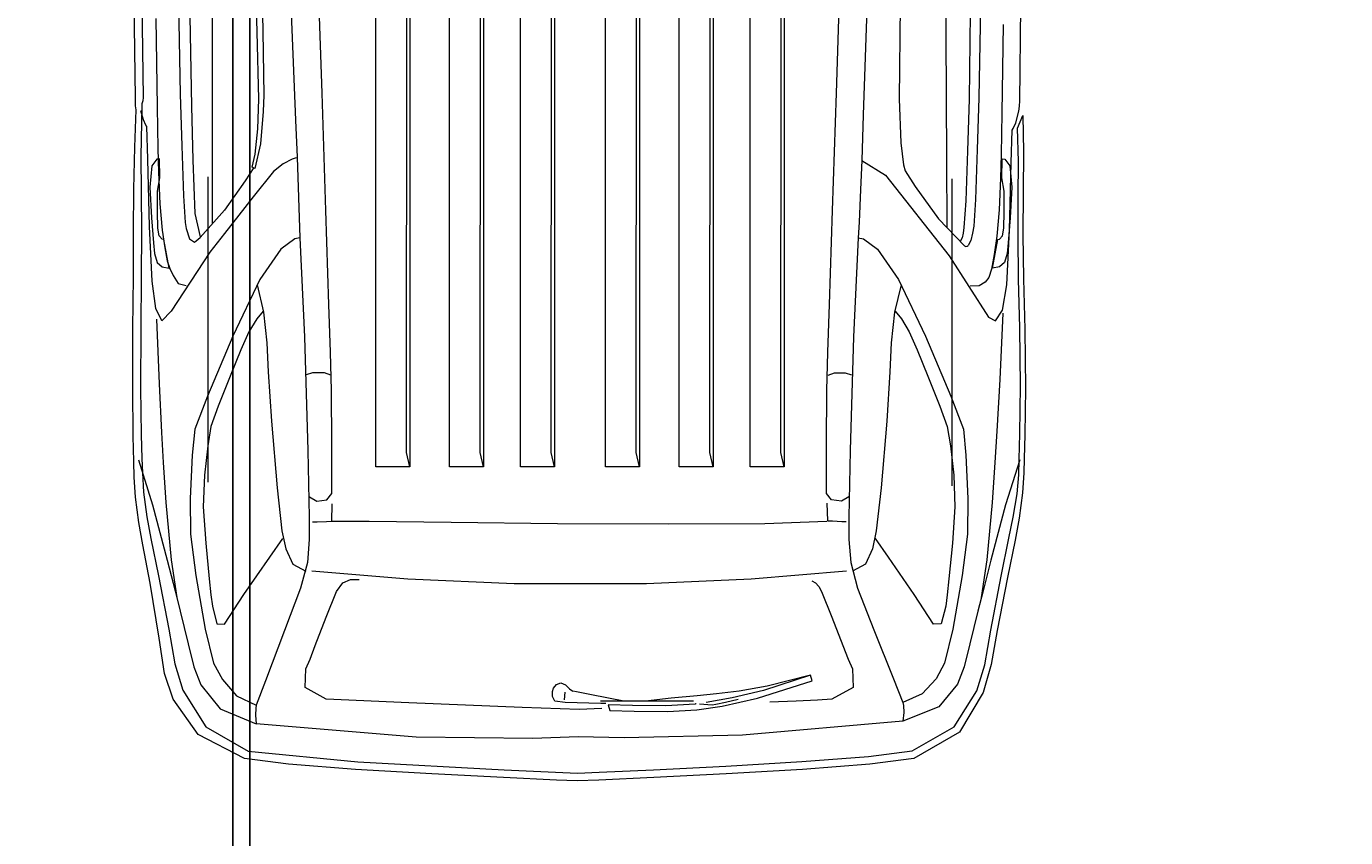
# Model space of a CAD drawing. Units: inches. Extents: x -10 to 502, y -868 to 56.
# Tile 3 of 14: x 78 to 165, y -724 to -671. Entities that reach past the tile are written whole.
import ezdxf

# ---------------------------------------------------------------- set-up
doc = ezdxf.new("R2010")
doc.units = ezdxf.units.IN
doc.header["$MEASUREMENT"] = 0
doc.layers.add('A-ANNO-DIMS', color=2, linetype='Continuous', lineweight=18)
doc.layers.add('C-PRKG-VEHI', color=8, linetype='Continuous', lineweight=13)
doc.styles.get("Standard").update_dxf_attribs({"font": 'arial.ttf'})
doc.dimstyles.get("Standard").update_dxf_attribs({"dimtxt": 0.18, "dimasz": 0.18, "dimexe": 0.18, "dimexo": 0.0625, "dimgap": 0.09, "dimtad": 0, "dimtih": 1, "dimtoh": 1, "dimdec": 0, "dimzin": 0, "dimdsep": 46, "dimlunit": 3, "dimtxsty": 'Standard', "dimcen": 0.09, "dimadec": 0, "dimazin": 0, "dimtfac": 1, "dimtdec": 0, "dimtofl": 0, "dimtmove": 0, "dimatfit": 3, "dimfxl": 1, "dimtolj": 1, "dimtzin": 0, "dimarcsym": 0})

# ---------------------------------------------------------------- blocks, each defined once
blk = doc.blocks.new('*D47')
at = {"layer": 'A-ANNO-DIMS', "color": 0, "lineweight": -2, "transparency": 16777216}
for p, q in [((91.951, -494.915), (91.951, -846.583)), ((201.951, -494.915), (201.951, -846.583)), ((92.131, -846.403), (146.622, -846.403)), ((201.771, -846.403), (147.28, -846.403))]:
    blk.add_line(p, q, dxfattribs=at)
at = {"layer": 'A-ANNO-DIMS', "color": 0, "transparency": 16777216}
for points in [[(92.131, -846.373), (92.131, -846.433), (91.951, -846.403)], [(201.771, -846.373), (201.771, -846.433), (201.951, -846.403)]]:
    blk.add_solid(points, dxfattribs=at)
at = {"layer": 'Defpoints', "color": 0, "transparency": 16777216}
for p in [(91.951, -494.853), (201.951, -494.853), (201.951, -846.403)]:
    blk.add_point(p, dxfattribs=at)
at = {"layer": 'A-ANNO-DIMS', "color": 0, "transparency": 16777216, "insert": (146.951, -846.403), "char_height": 0.18, "attachment_point": 5}
blk.add_mtext('\\A1;9\'-2"', dxfattribs=at)
blk = doc.blocks.new('*D56')
at = {"layer": 'A-ANNO-DIMS', "color": 0, "lineweight": -2, "transparency": 16777216}
for p, q in [((43.951, -549.915), (43.951, -846.583)), ((93.073, -549.915), (93.073, -846.583)), ((44.131, -846.403), (68.179, -846.403)), ((92.893, -846.403), (68.845, -846.403))]:
    blk.add_line(p, q, dxfattribs=at)
at = {"layer": 'A-ANNO-DIMS', "color": 0, "transparency": 16777216}
for points in [[(44.131, -846.373), (44.131, -846.433), (43.951, -846.403)], [(92.893, -846.373), (92.893, -846.433), (93.073, -846.403)]]:
    blk.add_solid(points, dxfattribs=at)
at = {"layer": 'Defpoints', "color": 0, "transparency": 16777216}
for p in [(43.951, -549.853), (93.073, -549.853), (43.951, -846.403)]:
    blk.add_point(p, dxfattribs=at)
at = {"layer": 'A-ANNO-DIMS', "color": 0, "transparency": 16777216, "insert": (68.512, -846.403), "char_height": 0.18, "attachment_point": 5}
blk.add_mtext('\\A1;4\'-1"', dxfattribs=at)
blk = doc.blocks.new('*D66')
at = {"layer": 'A-ANNO-DIMS', "color": 0, "lineweight": -2, "transparency": 16777216}
for p, q in [((217.361, -671.206), (217.541, -671.206)), ((217.451, -671.296), (217.451, -671.116)), ((144.253, -867.86), (171.639, -794.283)), ((144.073, -867.86), (144.253, -867.86))]:
    blk.add_line(p, q, dxfattribs=at)
at = {"layer": 'A-ANNO-DIMS', "color": 0, "transparency": 16777216}
blk.add_solid([(171.611, -794.273), (171.667, -794.294), (171.702, -794.115)], dxfattribs=at)
at = {"layer": 'Defpoints', "color": 0, "transparency": 16777216}
for p in [(217.451, -671.206), (171.702, -794.115)]:
    blk.add_point(p, dxfattribs=at)
at = {"layer": 'A-ANNO-DIMS', "color": 0, "transparency": 16777216, "insert": (143.323, -867.86), "char_height": 0.18, "attachment_point": 5}
blk.add_mtext('\\A1;2X R10\'-11"', dxfattribs=at)

msp = doc.modelspace()

# ---------------------------------------------------------------- linework, layer by layer
at = {"layer": 'C-PRKG-VEHI'}
for p, q in [((101.378, -699.991), (101.378, -640.902)), ((103.405, -699.052), (103.426, -641.088)), ((103.629, -640.902), (103.629, -699.991)), ((103.631, -640.902), (103.631, -699.991)), ((106.23, -699.991), (106.23, -640.902)), ((108.257, -699.052), (108.278, -641.088)), ((108.481, -640.902), (108.481, -699.991)), ((108.483, -640.902), (108.483, -699.991)), ((110.909, -699.991), (110.909, -640.902)), ((112.935, -699.052), (112.957, -641.088)), ((113.159, -640.902), (113.159, -699.991)), ((113.161, -640.902), (113.161, -699.991)), ((116.506, -699.991), (116.506, -640.902)), ((118.533, -699.052), (118.555, -641.088)), ((118.757, -640.902), (118.757, -699.991)), ((118.759, -640.902), (118.759, -699.991)), ((121.358, -699.991), (121.358, -640.902)), ((123.385, -699.052), (123.407, -641.088)), ((123.609, -640.902), (123.609, -699.991)), ((123.611, -640.902), (123.611, -699.991)), ((126.037, -699.991), (126.037, -640.902)), ((128.065, -699.052), (128.087, -641.088)), ((128.29, -640.902), (128.29, -699.991)), ((90.578, -659.407), (90.594, -671.12)), ((138.898, -663.527), (138.935, -671.511)), ((93.57, -671.36), (93.385, -665.39)), ((93.816, -665.754), (93.941, -671.332)), ((97.837, -675.397), (97.591, -667.668)), ((131.719, -675.397), (131.965, -667.668)), ((85.54, -675.7), (85.457, -669.432)), ((85.977, -669.417), (86.06, -675.679)), ((88.388, -669.553), (88.484, -675.465)), ((133.76, -669.192), (133.495, -676.811)), ((135.93, -669.616), (135.856, -675.761)), ((141.221, -669.747), (141.113, -675.705)), ((143.797, -675.928), (143.88, -669.667)), ((86.89, -670.481), (86.986, -676.312)), ((89.118, -670.332), (89.235, -676.238)), ((95.805, -670.125), (96.096, -677.158)), ((140.529, -670.12), (140.463, -675.791)), ((142.714, -670.872), (142.618, -676.703)), ((90.594, -671.12), (90.604, -679.492)), ((93.676, -675.783), (93.57, -671.36)), ((93.941, -671.332), (94, -675.532)), ((138.935, -671.511), (138.971, -679.778)), ((85.548, -675.964), (85.54, -675.7)), ((85.56, -676.228), (85.548, -675.964)), ((85.97, -676.087), (85.965, -676.303)), ((86.029, -675.896), (85.97, -676.087)), ((86.06, -675.679), (86.029, -675.896)), ((88.484, -675.465), (88.596, -678.86)), ((93.61, -677.738), (93.676, -675.783)), ((94, -675.532), (93.962, -676.596)), ((98.083, -683.122), (97.837, -675.397)), ((131.473, -683.122), (131.719, -675.397)), ((135.856, -675.761), (135.958, -678.658)), ((140.463, -675.791), (140.351, -679.186)), ((141.113, -675.705), (141.001, -679.099)), ((143.781, -676.195), (143.797, -675.928)), ((85.5, -678.937), (85.593, -676.491)), ((85.593, -676.491), (85.56, -676.228)), ((86.067, -677.15), (85.896, -676.543)), ((85.965, -676.303), (85.943, -677.321)), ((86.986, -676.312), (87.03, -679.044)), ((89.235, -676.238), (89.32, -679.804)), ((93.962, -676.596), (93.794, -678.731)), ((133.495, -676.811), (133.396, -679.829)), ((142.618, -676.703), (142.574, -679.435)), ((143.549, -677.34), (143.724, -676.661)), ((143.647, -677.689), (144.003, -676.854)), ((143.724, -676.661), (143.756, -676.439)), ((143.756, -676.439), (143.781, -676.195)), ((144.003, -676.854), (144.056, -679.247)), ((85.943, -677.321), (85.894, -679.549)), ((86.23, -677.487), (86.067, -677.15)), ((86.303, -677.59), (86.23, -677.487)), ((86.353, -679.745), (86.303, -677.59)), ((93.433, -679.404), (93.61, -677.738)), ((96.096, -677.158), (96.202, -679.604)), ((143.244, -679.984), (143.294, -677.83)), ((143.294, -677.83), (143.374, -677.715)), ((143.374, -677.715), (143.549, -677.34)), ((143.708, -679.887), (143.647, -677.689)), ((93.794, -678.731), (93.416, -680.353)), ((135.958, -678.658), (136.146, -680.114)), ((85.444, -681.703), (85.5, -678.937)), ((85.894, -679.549), (85.92, -681.916)), ((87.03, -679.044), (87.065, -680.598)), ((88.596, -678.86), (88.708, -682.156)), ((90.604, -679.492), (90.609, -683.966)), ((93.243, -680.266), (93.433, -679.404)), ((96.202, -679.604), (96.374, -684.912)), ((140.351, -679.186), (140.239, -682.481)), ((141.001, -679.099), (140.889, -682.395)), ((142.574, -679.435), (142.539, -680.989)), ((144.056, -679.247), (144.037, -681.916)), ((86.477, -684.16), (86.353, -679.745)), ((86.633, -680.175), (86.493, -681.579)), ((86.948, -679.731), (86.633, -680.175)), ((87.123, -679.703), (86.948, -679.731)), ((87.155, -680.958), (87.123, -679.703)), ((89.32, -679.804), (89.456, -683.311)), ((93.349, -680.275), (92.772, -681.168)), ((93.416, -680.353), (93.243, -680.266)), ((95.276, -680.041), (94.636, -680.555)), ((95.871, -679.742), (95.276, -680.041)), ((96.133, -679.645), (95.871, -679.742)), ((133.396, -679.829), (133.311, -681.722)), ((133.396, -679.829), (134.961, -680.794)), ((136.146, -680.114), (136.247, -680.514)), ((138.971, -679.778), (138.988, -684.205)), ((142.619, -680.958), (142.65, -679.703)), ((142.65, -679.703), (142.825, -679.731)), ((142.825, -679.731), (143.141, -680.175)), ((143.12, -684.4), (143.244, -679.984)), ((143.141, -680.175), (143.28, -681.579)), ((143.704, -682.199), (143.708, -679.887)), ((86.996, -681.836), (87.155, -680.958)), ((87.065, -680.598), (87.163, -682.673)), ((90.317, -680.894), (90.317, -700.996)), ((92.772, -681.168), (91.406, -683.09)), ((94.636, -680.555), (93.3, -682.205)), ((134.961, -680.794), (139.155, -686.106)), ((136.247, -680.514), (136.914, -681.541)), ((139.317, -681.039), (139.317, -701.249)), ((142.539, -680.989), (142.442, -683.064)), ((142.777, -681.836), (142.619, -680.958)), ((85.425, -684.518), (85.444, -681.703)), ((85.92, -681.916), (85.945, -684.518)), ((86.493, -681.579), (86.596, -683.597)), ((86.99, -683.197), (86.996, -681.836)), ((88.708, -682.156), (88.82, -683.91)), ((93.3, -682.205), (91.405, -684.626)), ((133.311, -681.722), (133.214, -683.882)), ((136.914, -681.541), (138.451, -683.662)), ((142.784, -683.197), (142.777, -681.836)), ((143.28, -681.579), (143.177, -683.597)), ((143.69, -684.772), (143.704, -682.199)), ((144.037, -681.916), (144.015, -684.685)), ((87.163, -682.673), (87.31, -684.413)), ((140.239, -682.481), (140.127, -684.236)), ((140.889, -682.395), (140.777, -684.149)), ((142.442, -683.064), (142.295, -684.804)), ((86.596, -683.597), (86.733, -685.251)), ((87.015, -684.274), (86.99, -683.197)), ((88.82, -683.91), (88.893, -684.305)), ((89.456, -683.311), (89.799, -684.859)), ((91.406, -683.09), (89.802, -684.9)), ((98.285, -689.315), (98.083, -683.122)), ((131.271, -689.315), (131.473, -683.122)), ((133.214, -683.882), (133.167, -684.912)), ((138.451, -683.662), (140.162, -685.435)), ((142.759, -684.274), (142.784, -683.197)), ((143.177, -683.597), (143.04, -685.251)), ((85.41, -687.487), (85.425, -684.518)), ((85.945, -684.518), (85.93, -687.487)), ((86.639, -687.769), (86.477, -684.16)), ((87.116, -684.788), (87.015, -684.274)), ((87.304, -684.994), (87.116, -684.788)), ((87.31, -684.413), (87.478, -685.575)), ((88.893, -684.305), (89.104, -684.985)), ((91.405, -684.626), (90.442, -685.867)), ((140.07, -684.6), (140.014, -684.917)), ((140.127, -684.236), (140.07, -684.6)), ((140.688, -684.604), (140.571, -685.089)), ((140.777, -684.149), (140.688, -684.604)), ((142.295, -684.804), (142.119, -686.018)), ((142.47, -684.994), (142.657, -684.788)), ((142.657, -684.788), (142.759, -684.274)), ((142.958, -688.008), (143.12, -684.4)), ((143.729, -687.633), (143.69, -684.772)), ((144.015, -684.685), (144.056, -687.611)), ((86.733, -685.251), (86.802, -685.937)), ((87.405, -685.032), (87.304, -684.994)), ((87.773, -686.916), (87.405, -685.032)), ((87.478, -685.575), (87.645, -686.439)), ((89.104, -684.985), (89.435, -685.196)), ((89.435, -685.196), (89.555, -685.107)), ((89.555, -685.107), (89.677, -685.007)), ((89.677, -685.007), (89.802, -684.9)), ((95.115, -685.654), (93.73, -687.669)), ((96.038, -684.977), (95.115, -685.654)), ((96.374, -684.912), (96.038, -684.977)), ((96.374, -684.912), (96.684, -691.432)), ((133.167, -684.912), (132.856, -691.432)), ((133.167, -684.912), (133.502, -684.977)), ((133.502, -684.977), (134.425, -685.654)), ((134.425, -685.654), (135.811, -687.669)), ((140.014, -684.917), (139.878, -685.162)), ((140.162, -685.435), (140.252, -685.477)), ((140.252, -685.477), (140.332, -685.472)), ((140.332, -685.472), (140.402, -685.425)), ((140.571, -685.089), (140.402, -685.425)), ((142, -686.916), (142.368, -685.032)), ((142.368, -685.032), (142.47, -684.994)), ((143.04, -685.251), (142.972, -685.937)), ((86.802, -685.937), (86.977, -686.541)), ((86.977, -686.541), (87.315, -686.831)), ((87.645, -686.439), (87.813, -686.93)), ((90.442, -685.867), (87.893, -689.754)), ((139.155, -686.106), (141.74, -690.144)), ((142.119, -686.018), (141.937, -686.979)), ((142.796, -686.541), (142.459, -686.831)), ((142.972, -685.937), (142.796, -686.541)), ((87.315, -686.831), (87.773, -686.916)), ((87.813, -686.93), (88.022, -687.391)), ((88.022, -687.391), (88.358, -687.912)), ((141.937, -686.979), (141.762, -687.523)), ((142.459, -686.831), (142, -686.916)), ((85.383, -690.907), (85.41, -687.487)), ((85.93, -687.487), (85.903, -690.907)), ((86.879, -689.575), (86.639, -687.769)), ((88.358, -687.912), (88.889, -688.043)), ((93.73, -687.669), (91.959, -691.384)), ((93.561, -688.006), (93.988, -689.806)), ((135.98, -688.006), (135.553, -689.806)), ((135.811, -687.669), (137.582, -691.384)), ((141.118, -688.066), (140.527, -688.108)), ((141.521, -687.823), (141.118, -688.066)), ((141.762, -687.523), (141.521, -687.823)), ((142.659, -689.687), (142.958, -688.008)), ((143.802, -690.851), (143.729, -687.633)), ((144.056, -687.611), (144.131, -690.95)), ((87.287, -690.369), (86.879, -689.575)), ((87.893, -689.754), (87.287, -690.369)), ((93.955, -689.75), (93.538, -690.257)), ((93.988, -689.806), (94.203, -691.832)), ((98.399, -692.45), (98.285, -689.315)), ((131.157, -692.45), (131.271, -689.315)), ((135.553, -689.806), (135.338, -691.832)), ((135.586, -689.75), (136.003, -690.257)), ((142.202, -690.387), (142.659, -689.687)), ((142.693, -689.884), (142.495, -694.244)), ((85.369, -694.813), (85.383, -690.907)), ((85.903, -690.907), (85.889, -694.813)), ((86.939, -690.274), (87.114, -694.532)), ((93.538, -690.257), (93.021, -691.1)), ((136.003, -690.257), (136.519, -691.1)), ((141.74, -690.144), (142.202, -690.387)), ((143.841, -694.649), (143.802, -690.851)), ((91.959, -691.384), (90.288, -695.336)), ((93.021, -691.1), (92.492, -692.282)), ((96.684, -691.432), (96.907, -698.927)), ((132.856, -691.432), (132.633, -698.927)), ((136.519, -691.1), (137.049, -692.282)), ((137.582, -691.384), (139.253, -695.336)), ((144.131, -690.95), (144.172, -694.813)), ((92.492, -692.282), (91.794, -694.032)), ((94.203, -691.832), (94.292, -693.745)), ((98.462, -694.975), (98.399, -692.45)), ((131.094, -694.975), (131.157, -692.45)), ((135.338, -691.832), (135.248, -693.745)), ((137.049, -692.282), (137.747, -694.032)), ((91.794, -694.032), (90.996, -696.007)), ((94.292, -693.745), (94.501, -696.983)), ((96.817, -693.913), (97.226, -693.781)), ((97.226, -693.781), (97.985, -693.788)), ((97.985, -693.788), (98.387, -693.945)), ((131.571, -693.831), (131.169, -693.988)), ((132.33, -693.825), (131.571, -693.831)), ((132.739, -693.956), (132.33, -693.825)), ((135.248, -693.745), (135.04, -696.983)), ((137.747, -694.032), (138.545, -696.007)), ((142.495, -694.244), (142.292, -697.636)), ((85.394, -697.97), (85.369, -694.813)), ((85.889, -694.813), (85.918, -697.895)), ((87.114, -694.532), (87.273, -697.737)), ((98.491, -698.498), (98.462, -694.975)), ((131.065, -698.498), (131.094, -694.975)), ((143.813, -697.809), (143.841, -694.649)), ((144.172, -694.813), (144.143, -697.895)), ((90.288, -695.336), (89.454, -697.514)), ((90.996, -696.007), (90.523, -697.345)), ((138.545, -696.007), (139.018, -697.345)), ((139.253, -695.336), (140.086, -697.514)), ((94.501, -696.983), (94.872, -701.383)), ((135.04, -696.983), (134.669, -701.383)), ((87.273, -697.737), (87.373, -699.708)), ((89.454, -697.514), (89.281, -699.233)), ((90.523, -697.345), (90.304, -698.604)), ((139.018, -697.345), (139.236, -698.604)), ((140.086, -697.514), (140.259, -699.233)), ((142.292, -697.636), (142.168, -699.708)), ((143.761, -699.497), (143.813, -697.809)), ((85.441, -699.652), (85.394, -697.97)), ((85.918, -697.895), (85.972, -699.439)), ((90.304, -698.604), (90.086, -700.55)), ((98.493, -701.748), (98.491, -698.498)), ((131.064, -701.748), (131.065, -698.498)), ((139.236, -698.604), (139.455, -700.55)), ((144.143, -697.895), (144.089, -699.439)), ((85.741, -699.539), (86.668, -702.496)), ((85.972, -699.439), (86.001, -700.383)), ((89.281, -699.233), (89.158, -702.077)), ((96.907, -698.927), (96.993, -703.309)), ((103.629, -699.991), (103.405, -699.052)), ((108.481, -699.991), (108.257, -699.052)), ((113.159, -699.991), (112.935, -699.052)), ((118.757, -699.991), (118.533, -699.052)), ((123.609, -699.991), (123.385, -699.052)), ((128.29, -699.991), (128.065, -699.052)), ((132.633, -698.927), (132.548, -703.309)), ((140.259, -699.233), (140.382, -702.077)), ((143.8, -699.539), (142.872, -702.496)), ((143.733, -700.519), (143.761, -699.497)), ((144.089, -699.439), (144.059, -700.383)), ((85.466, -700.671), (85.441, -699.652)), ((86.001, -700.383), (86.083, -701.661)), ((87.373, -699.708), (87.556, -702.35)), ((103.631, -699.991), (101.378, -699.991)), ((108.483, -699.991), (106.23, -699.991)), ((113.161, -699.991), (110.909, -699.991)), ((118.759, -699.991), (116.506, -699.991)), ((123.611, -699.991), (121.358, -699.991)), ((128.29, -699.991), (126.037, -699.991)), ((142.168, -699.708), (141.985, -702.35)), ((144.059, -700.383), (143.975, -701.706)), ((85.551, -701.993), (85.466, -700.671)), ((90.086, -700.55), (90.017, -702.633)), ((139.455, -700.55), (139.524, -702.633)), ((143.626, -701.759), (143.733, -700.519)), ((85.762, -703.651), (85.551, -701.993)), ((86.083, -701.661), (86.289, -703.278)), ((89.158, -702.077), (89.173, -704.434)), ((94.872, -701.383), (95.193, -704.209)), ((97.015, -701.964), (97.498, -702.256)), ((97.498, -702.256), (98.16, -702.162)), ((98.16, -702.162), (98.493, -701.748)), ((131.397, -702.162), (131.064, -701.748)), ((132.058, -702.256), (131.397, -702.162)), ((132.541, -701.964), (132.058, -702.256)), ((134.669, -701.383), (134.348, -704.209)), ((140.382, -702.077), (140.368, -704.434)), ((143.375, -703.305), (143.626, -701.759)), ((143.975, -701.706), (143.764, -703.363)), ((86.668, -702.496), (87.646, -706.128)), ((87.556, -702.35), (87.902, -706.105)), ((90.017, -702.633), (90.173, -705.011)), ((98.493, -702.436), (98.456, -703.59)), ((131.097, -702.388), (131.134, -703.542)), ((139.524, -702.633), (139.368, -705.011)), ((141.985, -702.35), (141.639, -706.105)), ((142.872, -702.496), (141.895, -706.128)), ((86.036, -705.119), (85.762, -703.651)), ((86.289, -703.278), (86.557, -704.711)), ((96.993, -703.309), (96.997, -704.769)), ((97.514, -703.631), (97.218, -703.646)), ((98.122, -703.604), (97.514, -703.631)), ((98.456, -703.59), (98.122, -703.604)), ((100.953, -703.601), (98.456, -703.59)), ((106.346, -703.665), (100.953, -703.601)), ((113.346, -703.737), (106.346, -703.665)), ((120.663, -703.777), (113.346, -703.737)), ((127.006, -703.742), (120.663, -703.777)), ((131.085, -703.59), (127.006, -703.742)), ((131.134, -703.542), (131.468, -703.556)), ((131.468, -703.556), (132.076, -703.584)), ((132.076, -703.584), (132.372, -703.598)), ((132.548, -703.309), (132.544, -704.769)), ((143.083, -704.699), (143.375, -703.305)), ((143.764, -703.363), (143.49, -704.831)), ((86.557, -704.711), (87.067, -707.174)), ((89.173, -704.434), (89.529, -707.136)), ((94.394, -705.936), (95.249, -704.715)), ((95.193, -704.209), (95.451, -705.382)), ((96.997, -704.769), (96.876, -706.292)), ((132.544, -704.769), (132.665, -706.292)), ((134.348, -704.209), (134.09, -705.382)), ((135.146, -705.936), (134.292, -704.715)), ((140.368, -704.434), (140.012, -707.136)), ((142.573, -707.188), (143.083, -704.699)), ((86.507, -707.641), (86.036, -705.119)), ((90.173, -705.011), (90.404, -707.363)), ((95.451, -705.382), (95.909, -706.392)), ((134.09, -705.382), (133.632, -706.392)), ((139.368, -705.011), (139.136, -707.363)), ((143.49, -704.831), (142.983, -707.278)), ((87.646, -706.128), (88.16, -708.147)), ((87.902, -706.105), (88.273, -708.597)), ((92.69, -708.407), (94.394, -705.936)), ((95.909, -706.392), (96.768, -706.853)), ((96.876, -706.292), (96.43, -707.978)), ((132.665, -706.292), (133.11, -707.978)), ((133.632, -706.392), (132.773, -706.853)), ((136.851, -708.407), (135.146, -705.936)), ((141.639, -706.105), (141.268, -708.597)), ((141.895, -706.128), (141.38, -708.147)), ((87.067, -707.174), (87.74, -710.678)), ((89.529, -707.136), (90.148, -710.676)), ((90.404, -707.363), (90.523, -708.428)), ((103.494, -707.384), (97.161, -706.853)), ((99.198, -707.64), (99.712, -707.419)), ((99.712, -707.419), (100.281, -707.413)), ((110.501, -707.69), (103.494, -707.384)), ((126.105, -707.384), (119.206, -707.69)), ((132.379, -706.853), (126.105, -707.384)), ((139.136, -707.363), (139.018, -708.428)), ((140.012, -707.136), (139.393, -710.676)), ((141.899, -710.739), (142.573, -707.188)), ((142.983, -707.278), (142.314, -710.758)), ((87.11, -711.263), (86.507, -707.641)), ((88.16, -708.147), (88.494, -709.495)), ((96.43, -707.978), (95.372, -710.774)), ((98.116, -709.88), (98.793, -708.203)), ((98.793, -708.203), (99.198, -707.64)), ((114.883, -707.696), (110.501, -707.69)), ((119.206, -707.69), (114.883, -707.696)), ((130.094, -707.494), (130.342, -707.639)), ((130.342, -707.639), (130.562, -707.87)), ((130.562, -707.87), (130.748, -708.203)), ((130.748, -708.203), (131.425, -709.88)), ((133.11, -707.978), (134.188, -710.729)), ((141.38, -708.147), (141.047, -709.495)), ((90.523, -708.428), (90.619, -709.161)), ((91.423, -710.341), (92.69, -708.407)), ((138.118, -710.341), (136.851, -708.407)), ((139.018, -708.428), (138.922, -709.161)), ((88.494, -709.495), (89.027, -711.655)), ((90.619, -709.161), (90.915, -710.32)), ((97.389, -711.758), (98.116, -709.88)), ((131.425, -709.88), (132.152, -711.758)), ((138.922, -709.161), (138.626, -710.32)), ((141.047, -709.495), (140.514, -711.655)), ((87.74, -710.678), (88.137, -712.953)), ((90.148, -710.676), (90.692, -712.928)), ((90.915, -710.32), (91.423, -710.341)), ((95.372, -710.774), (94.113, -714.082)), ((134.188, -710.729), (135.481, -713.954)), ((138.626, -710.32), (138.118, -710.341)), ((139.393, -710.676), (138.849, -712.928)), ((141.502, -713.039), (141.899, -710.739)), ((142.314, -710.758), (141.92, -713.017)), ((87.469, -713.598), (87.11, -711.263)), ((89.027, -711.655), (89.398, -713.153)), ((97.049, -712.647), (97.389, -711.758)), ((132.152, -711.758), (132.492, -712.647)), ((140.514, -711.655), (140.143, -713.153)), ((88.137, -712.953), (88.666, -714.69)), ((89.398, -713.153), (89.859, -714.341)), ((90.692, -712.928), (91.271, -713.991)), ((96.716, -714.531), (96.763, -713.295)), ((96.763, -713.295), (97.049, -712.647)), ((132.492, -712.647), (132.777, -713.295)), ((132.777, -713.295), (132.825, -714.531)), ((138.849, -712.928), (138.288, -713.947)), ((140.143, -713.153), (139.701, -714.296)), ((140.983, -714.749), (141.502, -713.039)), ((141.92, -713.017), (141.401, -714.852)), ((88.027, -715.283), (87.469, -713.598)), ((89.859, -714.341), (91.12, -715.915)), ((91.271, -713.991), (92.213, -715.065)), ((94.113, -714.082), (93.505, -715.678)), ((113.077, -714.575), (113.279, -714.321)), ((113.279, -714.321), (113.56, -714.208)), ((113.56, -714.208), (113.87, -714.35)), ((113.87, -714.35), (114.15, -714.603)), ((126.522, -715.232), (130.131, -714.083)), ((130.017, -713.709), (126.913, -714.71)), ((130.017, -713.709), (127.162, -714.426)), ((130.131, -714.083), (130.017, -713.709)), ((135.481, -713.954), (136.109, -715.505)), ((138.288, -713.947), (137.382, -714.937)), ((139.701, -714.296), (138.475, -715.787)), ((88.666, -714.69), (90.193, -717.111)), ((92.213, -715.065), (93.505, -715.678)), ((98.118, -715.291), (96.716, -714.531)), ((113.019, -714.793), (113.077, -714.575)), ((113.029, -715.121), (113.019, -714.793)), ((113.175, -715.41), (113.029, -715.121)), ((113.808, -715.332), (113.844, -714.823)), ((114.15, -714.603), (114.354, -714.759)), ((114.604, -714.802), (114.354, -714.759)), ((115.6, -714.993), (114.604, -714.802)), ((117.717, -715.424), (115.6, -714.993)), ((120.845, -715.221), (119.136, -715.42)), ((122.547, -715.066), (120.845, -715.221)), ((123.813, -714.944), (122.547, -715.066)), ((124.849, -715.205), (123.144, -715.501)), ((125.309, -714.761), (123.813, -714.944)), ((124.194, -715.757), (126.522, -715.232)), ((126.913, -714.71), (124.849, -715.205)), ((127.162, -714.426), (125.309, -714.761)), ((132.825, -714.531), (131.423, -715.291)), ((137.382, -714.937), (136.109, -715.505)), ((139.474, -717.118), (140.983, -714.749)), ((141.401, -714.852), (139.824, -717.459)), ((89.677, -717.609), (88.027, -715.283)), ((91.12, -715.915), (93.505, -716.916)), ((93.48, -715.874), (93.455, -716.345)), ((93.505, -715.678), (93.48, -715.874)), ((103.56, -715.541), (98.118, -715.291)), ((111.016, -715.829), (103.56, -715.541)), ((114.77, -715.967), (111.016, -715.829)), ((113.849, -715.513), (113.175, -715.41)), ((116.21, -715.571), (113.849, -715.513)), ((116.268, -715.912), (114.77, -715.967)), ((117.95, -715.42), (116.188, -715.411)), ((116.544, -715.574), (116.21, -715.571)), ((118.28, -715.716), (116.682, -715.667)), ((116.682, -715.667), (116.796, -716.041)), ((116.796, -716.041), (118.394, -716.09)), ((120.806, -715.427), (117.95, -715.42)), ((120.476, -715.717), (118.28, -715.716)), ((118.394, -716.09), (120.59, -716.091)), ((122.419, -715.609), (120.476, -715.717)), ((120.59, -716.091), (122.533, -715.982)), ((122.302, -715.43), (120.806, -715.427)), ((122.441, -715.606), (122.419, -715.609)), ((122.463, -715.603), (122.441, -715.606)), ((122.486, -715.6), (122.463, -715.603)), ((122.533, -715.982), (124.194, -715.757)), ((123.529, -715.68), (122.707, -715.618)), ((123.785, -715.632), (123.529, -715.68)), ((124.423, -715.501), (123.785, -715.632)), ((125.249, -715.308), (124.423, -715.501)), ((129.072, -715.411), (127.332, -715.486)), ((130.474, -715.345), (129.072, -715.411)), ((131.423, -715.291), (130.474, -715.345)), ((136.109, -715.505), (136.134, -715.701)), ((138.475, -715.787), (136.109, -716.743)), ((136.134, -715.701), (136.159, -716.172)), ((93.455, -716.345), (93.505, -716.916)), ((104.029, -717.787), (93.505, -716.916)), ((136.109, -716.743), (125.536, -717.658)), ((136.159, -716.172), (136.109, -716.743)), ((92.723, -719.203), (89.677, -717.609)), ((90.193, -717.111), (92.961, -718.714)), ((111.728, -717.871), (104.029, -717.787)), ((114.714, -717.767), (111.728, -717.871)), ((117.748, -717.826), (114.714, -717.767)), ((125.536, -717.658), (117.748, -717.826)), ((136.716, -718.693), (139.474, -717.118)), ((139.824, -717.459), (136.818, -719.203)), ((92.961, -718.714), (100.199, -719.409)), ((133.834, -719.054), (136.716, -718.693)), ((95.622, -719.567), (92.723, -719.203)), ((100.043, -719.911), (95.622, -719.567)), ((100.199, -719.409), (109.84, -719.939)), ((124.44, -719.694), (129.439, -719.394)), ((129.439, -719.394), (133.834, -719.054)), ((133.919, -719.567), (129.497, -719.911)), ((136.818, -719.203), (133.919, -719.567)), ((105.073, -720.213), (100.043, -719.911)), ((109.784, -720.454), (105.073, -720.213)), ((113.28, -720.613), (109.784, -720.454)), ((109.84, -719.939), (114.668, -720.151)), ((114.668, -720.151), (116.088, -720.094)), ((119.692, -720.454), (116.079, -720.613)), ((116.088, -720.094), (119.679, -719.935)), ((119.679, -719.935), (124.44, -719.694)), ((124.468, -720.213), (119.692, -720.454)), ((129.497, -719.911), (124.468, -720.213)), ((114.647, -720.671), (113.28, -720.613)), ((116.079, -720.613), (114.647, -720.671))]:
    msp.add_line(p, q, dxfattribs=at)

# ---------------------------------------------------------------- dimensions: what is measured, and where the dimension line sits
at = {"layer": 'A-ANNO-DIMS'}
for base, p1, p2, picture, middle in [((201.951, -846.403), (91.951, -494.853), (201.951, -494.853), '*D47', (146.951, -846.403)), ((43.951, -846.403), (93.073, -549.853), (43.951, -549.853), '*D56', (68.512, -846.403))]:
    dim = msp.add_linear_dim(base=base, p1=p1, p2=p2, dimstyle='Standard', override={"dimdec": 1, "dimlfac": 1, "dimrnd": 0, "dimzin": 1, "dimdsep": 46, "dimlunit": 4, "dimfrac": 2}, dxfattribs=at)
    dim.commit()
    dim.dimension.update_dxf_attribs({"geometry": picture, "text_midpoint": middle})
dim = msp.add_radius_dim(center=(217.451, -671.206), mpoint=(171.702, -794.115), text='2X <>', dimstyle='Standard', override={"dimdec": 1, "dimlfac": 1, "dimrnd": 0, "dimzin": 1, "dimdsep": 46, "dimlunit": 4, "dimfrac": 2}, dxfattribs=at)
dim.commit()
dim.dimension.update_dxf_attribs({"geometry": '*D66', "text_midpoint": (143.323, -867.86), "dimtype": 164})

doc.saveas('drawing.dxf')
